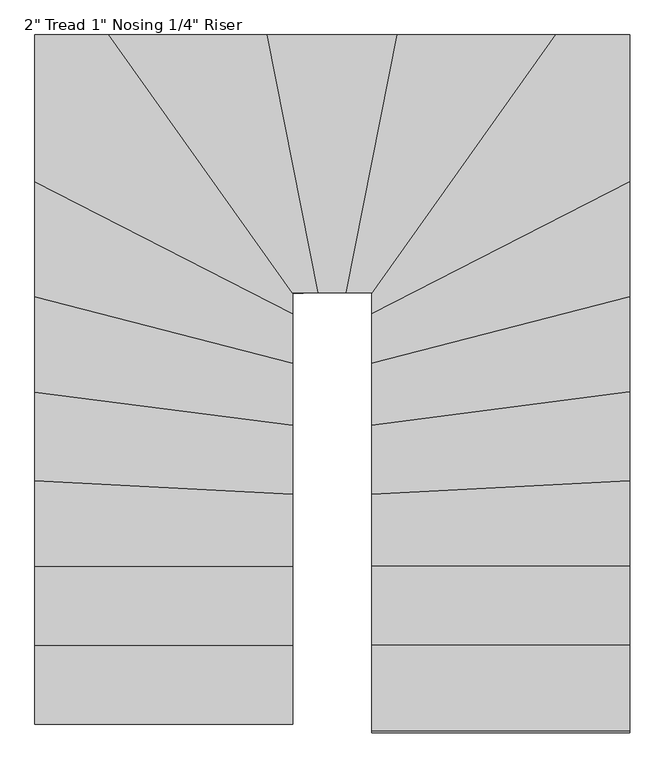
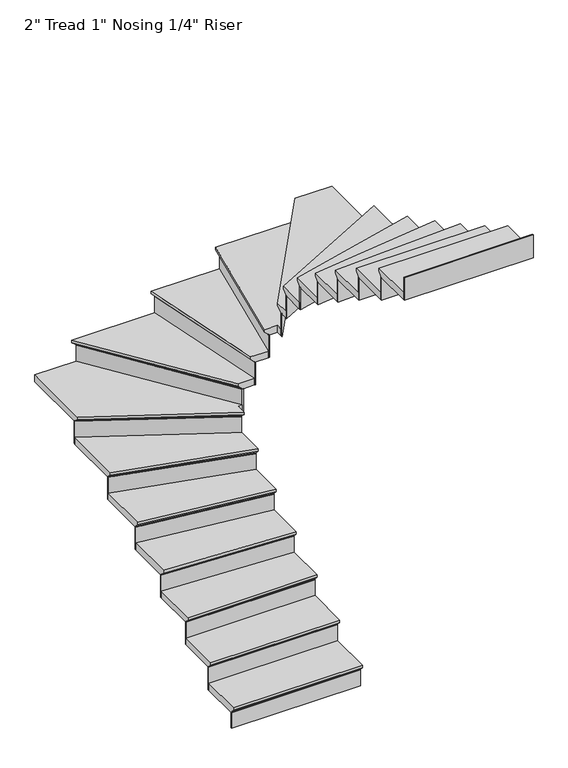
"""IFC4 building model written with IfcOpenShell, lengths in millimetres: stair flight geometry."""

from ifc_helpers import new_model, si_unit, origin, place, context, project, spatial, faceted_brep, source, transform, mapped, element, save


def stair_flight_f68c085a(model_context):
    return source(origin(), model_context, "Body", "Brep", [
        faceted_brep([(-12370.7568901, 792.321124, 150.2833333), (-12370.7568901, 792.321124, 169.3333333), (-13285.1568901, 792.321124, 169.3333333), (-13285.1568901, 792.321124, 150.2833333), (-12370.7568901, 817.721124, 124.8833333), (-13285.1568901, 817.721124, 124.8833333), (-12370.7568901, 1097.121124, 169.3333333), (-13285.1568901, 1097.121124, 169.3333333), (-13285.1568901, 817.721124, 118.5333333), (-13285.1568901, 1097.121124, 118.5333333), (-12370.7568901, 1097.121124, 118.5333333), (-12370.7568901, 817.721124, 118.5333333)], [[[0, 1, 2, 3]], [[4, 0, 3, 5]], [[2, 1, 6, 7]], [[8, 9, 10, 11]], [[2, 7, 9, 8, 5, 3]], [[8, 11, 4, 5]], [[6, 1, 0, 4, 11, 10]], [[7, 6, 10, 9]]]),
        faceted_brep([(-12370.7568901, 817.721124, 118.5333333), (-12370.7568901, 817.721124, 0.0), (-12370.7568901, 824.071124, 0.0), (-12370.7568901, 824.071124, 118.5333333), (-13285.1568901, 817.721124, 118.5333333), (-13285.1568901, 824.071124, 118.5333333), (-13285.1568901, 824.071124, 0.0), (-13285.1568901, 817.721124, 0.0)], [[[0, 1, 2, 3]], [[4, 5, 6, 7]], [[1, 0, 4, 7]], [[2, 1, 7, 6]], [[3, 2, 6, 5]], [[0, 3, 5, 4]]]),
        faceted_brep([(-12370.7568901, 1097.121124, 287.8666667), (-12370.7568901, 1097.121124, 118.5333333), (-12370.7568901, 1103.471124, 118.5333333), (-12370.7568901, 1103.471124, 287.8666667), (-13285.1568901, 1097.121124, 287.8666667), (-13285.1568901, 1103.471124, 287.8666667), (-13285.1568901, 1103.471124, 118.5333333), (-13285.1568901, 1097.121124, 118.5333333)], [[[0, 1, 2, 3]], [[4, 5, 6, 7]], [[1, 0, 4, 7]], [[2, 1, 7, 6]], [[3, 2, 6, 5]], [[0, 3, 5, 4]]]),
        faceted_brep([(-13285.1568901, 1071.721124, 338.6666667), (-12370.7568901, 1071.721124, 338.6666667), (-12370.7568901, 1376.521124, 338.6666667), (-13285.1568901, 1376.521124, 338.6666667), (-13285.1568901, 1097.121124, 287.8666667), (-13285.1568901, 1376.521124, 287.8666667), (-12370.7568901, 1376.521124, 287.8666667), (-12370.7568901, 1097.121124, 287.8666667), (-13285.1568901, 1097.121124, 294.2166667), (-13285.1568901, 1071.721124, 319.6166667), (-12370.7568901, 1097.121124, 294.2166667), (-12370.7568901, 1071.721124, 319.6166667)], [[[0, 1, 2, 3]], [[4, 5, 6, 7]], [[0, 3, 5, 4, 8, 9]], [[4, 7, 10, 8]], [[2, 1, 11, 10, 7, 6]], [[3, 2, 6, 5]], [[11, 1, 0, 9]], [[10, 11, 9, 8]]]),
        faceted_brep([(-12370.7568901, 1376.521124, 457.2), (-12370.7568901, 1376.521124, 287.8666667), (-12370.7568901, 1382.871124, 287.8666667), (-12370.7568901, 1382.871124, 457.2), (-13285.1568901, 1376.521124, 457.2), (-13285.1568901, 1382.871124, 457.2), (-13285.1568901, 1382.871124, 287.8666667), (-13285.1568901, 1376.521124, 287.8666667)], [[[0, 1, 2, 3]], [[4, 5, 6, 7]], [[1, 0, 4, 7]], [[2, 1, 7, 6]], [[3, 2, 6, 5]], [[0, 3, 5, 4]]]),
        faceted_brep([(-13285.1568901, 1351.121124, 508.0), (-12370.7568901, 1351.121124, 508.0), (-12370.7568901, 1632.1882855, 508.0), (-13285.1568901, 1679.7225559, 508.0), (-13285.1568901, 1376.521124, 457.2), (-13285.1568901, 1679.7225559, 457.2), (-12370.7568901, 1632.1882855, 457.2), (-12370.7568901, 1376.521124, 457.2), (-13285.1568901, 1376.521124, 463.55), (-13285.1568901, 1351.121124, 488.95), (-12370.7568901, 1376.521124, 463.55), (-12370.7568901, 1351.121124, 488.95)], [[[0, 1, 2, 3]], [[4, 5, 6, 7]], [[0, 3, 5, 4, 8, 9]], [[4, 7, 10, 8]], [[2, 1, 11, 10, 7, 6]], [[3, 2, 6, 5]], [[11, 1, 0, 9]], [[10, 11, 9, 8]]]),
        faceted_brep([(-12370.7568901, 1632.1882855, 626.5333333), (-12370.7568901, 1632.1882855, 457.2), (-12370.7568901, 1638.5468597, 457.2), (-12370.7568901, 1638.5468597, 626.5333333), (-13285.1568901, 1679.7225559, 626.5333333), (-13285.1568901, 1686.0811301, 626.5333333), (-13285.1568901, 1686.0811301, 457.2), (-13285.1568901, 1679.7225559, 457.2)], [[[0, 1, 2, 3]], [[4, 5, 6, 7]], [[1, 0, 4, 7]], [[2, 1, 7, 6]], [[3, 2, 6, 5]], [[0, 3, 5, 4]]]),
        faceted_brep([(-13285.1568901, 1654.2882592, 677.3333333), (-12370.7568901, 1606.7539888, 677.3333333), (-12370.7568901, 1876.3549853, 677.3333333), (-13285.1568901, 1994.711037, 677.3333333), (-13285.1568901, 1679.7225559, 626.5333333), (-13285.1568901, 1994.711037, 626.5333333), (-12370.7568901, 1876.3549853, 626.5333333), (-12370.7568901, 1632.1882855, 626.5333333), (-13285.1568901, 1679.7225559, 632.8833333), (-13285.1568901, 1654.2882592, 658.2833333), (-12370.7568901, 1632.1882855, 632.8833333), (-12370.7568901, 1606.7539888, 658.2833333)], [[[0, 1, 2, 3]], [[4, 5, 6, 7]], [[0, 3, 5, 4, 8, 9]], [[4, 7, 10, 8]], [[2, 1, 11, 10, 7, 6]], [[3, 2, 6, 5]], [[11, 1, 0, 9]], [[10, 11, 9, 8]]]),
        faceted_brep([(-12370.7568901, 1876.3549853, 795.8666667), (-12370.7568901, 1876.3549853, 626.5333333), (-12370.7568901, 1882.7579571, 626.5333333), (-12370.7568901, 1882.7579571, 795.8666667), (-13285.1568901, 1994.711037, 795.8666667), (-13285.1568901, 2001.1140088, 795.8666667), (-13285.1568901, 2001.1140088, 626.5333333), (-13285.1568901, 1994.711037, 626.5333333)], [[[0, 1, 2, 3]], [[4, 5, 6, 7]], [[1, 0, 4, 7]], [[2, 1, 7, 6]], [[3, 2, 6, 5]], [[0, 3, 5, 4]]]),
        faceted_brep([(-13285.1568901, 1969.0991499, 846.6666667), (-12370.7568901, 1850.7430982, 846.6666667), (-12370.7568901, 2097.9822078, 846.6666667), (-13285.1568901, 2333.1126552, 846.6666667), (-13285.1568901, 1994.711037, 795.8666667), (-13285.1568901, 2333.1126552, 795.8666667), (-12370.7568901, 2097.9822078, 795.8666667), (-12370.7568901, 1876.3549853, 795.8666667), (-13285.1568901, 1994.711037, 802.2166667), (-13285.1568901, 1969.0991499, 827.6166667), (-12370.7568901, 1876.3549853, 802.2166667), (-12370.7568901, 1850.7430982, 827.6166667)], [[[0, 1, 2, 3]], [[4, 5, 6, 7]], [[0, 3, 5, 4, 8, 9]], [[4, 7, 10, 8]], [[2, 1, 11, 10, 7, 6]], [[3, 2, 6, 5]], [[11, 1, 0, 9]], [[10, 11, 9, 8]]]),
        faceted_brep([(-12370.7568901, 2097.9822078, 965.2), (-12370.7568901, 2097.9822078, 795.8666667), (-12370.7568901, 2104.5387847, 795.8666667), (-12370.7568901, 2104.5387847, 965.2), (-13285.1568901, 2333.1126552, 965.2), (-13285.1568901, 2339.6692321, 965.2), (-13285.1568901, 2339.6692321, 795.8666667), (-13285.1568901, 2333.1126552, 795.8666667)], [[[0, 1, 2, 3]], [[4, 5, 6, 7]], [[1, 0, 4, 7]], [[2, 1, 7, 6]], [[3, 2, 6, 5]], [[0, 3, 5, 4]]]),
        faceted_brep([(-13285.1568901, 2306.8863477, 1016.0), (-12370.7568901, 2071.7559003, 1016.0), (-12370.7568901, 2274.3288439, 1016.0), (-13285.1568901, 2743.1534652, 1016.0), (-13285.1568901, 2333.1126552, 965.2), (-13285.1568901, 2743.1534652, 965.2), (-12370.7568901, 2274.3288439, 965.2), (-12370.7568901, 2097.9822078, 965.2), (-13285.1568901, 2333.1126552, 971.55), (-13285.1568901, 2306.8863477, 996.95), (-12370.7568901, 2097.9822078, 971.55), (-12370.7568901, 2071.7559003, 996.95)], [[[0, 1, 2, 3]], [[4, 5, 6, 7]], [[0, 3, 5, 4, 8, 9]], [[4, 7, 10, 8]], [[2, 1, 11, 10, 7, 6]], [[3, 2, 6, 5]], [[11, 1, 0, 9]], [[10, 11, 9, 8]]]),
        faceted_brep([(-12370.7568901, 2274.3288439, 1134.5333333), (-12370.7568901, 2274.3288439, 965.2), (-12370.7568901, 2281.464827, 965.2), (-12370.7568901, 2281.464827, 1134.5333333), (-13285.1568901, 2743.1534652, 1134.5333333), (-13285.1568901, 2750.2894483, 1134.5333333), (-13285.1568901, 2750.2894483, 965.2), (-13285.1568901, 2743.1534652, 965.2)], [[[0, 1, 2, 3]], [[4, 5, 6, 7]], [[1, 0, 4, 7]], [[2, 1, 7, 6]], [[3, 2, 6, 5]], [[0, 3, 5, 4]]]),
        faceted_brep([(-12991.4757564, 3234.4528159, 1185.3333333), (-13285.1568901, 3234.4528159, 1185.3333333), (-13285.1568901, 2714.6095327, 1185.3333333), (-12370.7568901, 2245.7849113, 1185.3333333), (-12370.7568901, 2320.0528159, 1185.3333333), (-12341.2018072, 2320.0528159, 1185.3333333), (-13285.1568901, 3234.4528159, 1134.5333333), (-12991.4757564, 3234.4528159, 1134.5333333), (-12341.2018072, 2320.0528159, 1134.5333333), (-12370.7568901, 2320.0528159, 1134.5333333), (-12370.7568901, 2274.3288439, 1134.5333333), (-13285.1568901, 2743.1534652, 1134.5333333), (-13285.1568901, 2743.1534652, 1140.8833333), (-13285.1568901, 2714.6095327, 1166.2833333), (-12370.7568901, 2274.3288439, 1140.8833333), (-12370.7568901, 2245.7849113, 1166.2833333)], [[[0, 1, 2, 3, 4, 5]], [[6, 7, 8, 9, 10, 11]], [[1, 0, 7, 6]], [[2, 1, 6, 11, 12, 13]], [[11, 10, 14, 12]], [[4, 3, 15, 14, 10, 9]], [[5, 4, 9, 8]], [[0, 5, 8, 7]], [[15, 3, 2, 13]], [[14, 15, 13, 12]]]),
        faceted_brep([(-12341.2018072, 2320.0528159, 1303.8666667), (-12341.2018072, 2320.0528159, 1134.5333333), (-12333.4098325, 2320.0528159, 1134.5333333), (-12333.4098325, 2320.0528159, 1303.8666667), (-12991.4757564, 3234.4528159, 1303.8666667), (-12983.6837816, 3234.4528159, 1303.8666667), (-12983.6837816, 3234.4528159, 1134.5333333), (-12991.4757564, 3234.4528159, 1134.5333333)], [[[0, 1, 2, 3]], [[4, 5, 6, 7]], [[1, 0, 4, 7]], [[2, 1, 7, 6]], [[3, 2, 6, 5]], [[0, 3, 5, 4]]]),
        faceted_brep([(-13022.6436556, 3234.4528159, 1354.6666667), (-12372.3697064, 2320.0528159, 1354.6666667), (-12254.7477202, 2320.0528159, 1354.6666667), (-12434.9885765, 3234.4528159, 1354.6666667), (-12991.4757564, 3234.4528159, 1303.8666667), (-12434.9885765, 3234.4528159, 1303.8666667), (-12254.7477202, 2320.0528159, 1303.8666667), (-12341.2018072, 2320.0528159, 1303.8666667), (-12991.4757564, 3234.4528159, 1310.2166667), (-13022.6436556, 3234.4528159, 1335.6166667), (-12341.2018072, 2320.0528159, 1310.2166667), (-12372.3697064, 2320.0528159, 1335.6166667)], [[[0, 1, 2, 3]], [[4, 5, 6, 7]], [[0, 3, 5, 4, 8, 9]], [[4, 7, 10, 8]], [[2, 1, 11, 10, 7, 6]], [[3, 2, 6, 5]], [[11, 1, 0, 9]], [[10, 11, 9, 8]]]),
        faceted_brep([(-12254.7477202, 2320.0528159, 1473.2), (-12254.7477202, 2320.0528159, 1303.8666667), (-12248.2755347, 2320.0528159, 1303.8666667), (-12248.2755347, 2320.0528159, 1473.2), (-12434.9885765, 3234.4528159, 1473.2), (-12428.5163911, 3234.4528159, 1473.2), (-12428.5163911, 3234.4528159, 1303.8666667), (-12434.9885765, 3234.4528159, 1303.8666667)], [[[0, 1, 2, 3]], [[4, 5, 6, 7]], [[1, 0, 4, 7]], [[2, 1, 7, 6]], [[3, 2, 6, 5]], [[0, 3, 5, 4]]]),
        faceted_brep([(-12460.8773183, 3234.4528159, 1524.0), (-12280.6364619, 2320.0528159, 1524.0), (-12155.5885765, 2320.0528159, 1524.0), (-11975.3477202, 3234.4528159, 1524.0), (-12434.9885765, 3234.4528159, 1473.2), (-11975.3477202, 3234.4528159, 1473.2), (-12155.5885765, 2320.0528159, 1473.2), (-12254.7477202, 2320.0528159, 1473.2), (-12434.9885765, 3234.4528159, 1479.55), (-12460.8773183, 3234.4528159, 1504.95), (-12254.7477202, 2320.0528159, 1479.55), (-12280.6364619, 2320.0528159, 1504.95)], [[[0, 1, 2, 3]], [[4, 5, 6, 7]], [[0, 3, 5, 4, 8, 9]], [[4, 7, 10, 8]], [[2, 1, 11, 10, 7, 6]], [[3, 2, 6, 5]], [[11, 1, 0, 9]], [[10, 11, 9, 8]]]),
        faceted_brep([(-12155.5885765, 2320.0528159, 1642.5333333), (-12155.5885765, 2320.0528159, 1473.2), (-12149.1163911, 2320.0528159, 1473.2), (-12149.1163911, 2320.0528159, 1642.5333333), (-11975.3477202, 3234.4528159, 1642.5333333), (-11968.8755347, 3234.4528159, 1642.5333333), (-11968.8755347, 3234.4528159, 1473.2), (-11975.3477202, 3234.4528159, 1473.2)], [[[0, 1, 2, 3]], [[4, 5, 6, 7]], [[1, 0, 4, 7]], [[2, 1, 7, 6]], [[3, 2, 6, 5]], [[0, 3, 5, 4]]]),
        faceted_brep([(-12001.2364619, 3234.4528159, 1693.3333333), (-12181.4773183, 2320.0528159, 1693.3333333), (-12091.3568901, 2320.0528159, 1693.3333333), (-12091.3568901, 2273.9573414, 1693.3333333), (-11408.3022254, 3234.4528159, 1693.3333333), (-11975.3477202, 3234.4528159, 1642.5333333), (-11408.3022254, 3234.4528159, 1642.5333333), (-12091.3568901, 2273.9573414, 1642.5333333), (-12091.3568901, 2320.0528159, 1642.5333333), (-12155.5885765, 2320.0528159, 1642.5333333), (-11975.3477202, 3234.4528159, 1648.8833333), (-12001.2364619, 3234.4528159, 1674.2833333), (-12155.5885765, 2320.0528159, 1648.8833333), (-12181.4773183, 2320.0528159, 1674.2833333)], [[[0, 1, 2, 3, 4]], [[5, 6, 7, 8, 9]], [[0, 4, 6, 5, 10, 11]], [[5, 9, 12, 10]], [[2, 1, 13, 12, 9, 8]], [[3, 2, 8, 7]], [[4, 3, 7, 6]], [[13, 1, 0, 11]], [[12, 13, 11, 10]]]),
        faceted_brep([(-12091.3568901, 2273.9573414, 1811.8666667), (-12091.3568901, 2273.9573414, 1642.5333333), (-12091.3568901, 2263.0004489, 1642.5333333), (-12091.3568901, 2263.0004489, 1811.8666667), (-11408.3022254, 3234.4528159, 1811.8666667), (-11400.5102506, 3234.4528159, 1811.8666667), (-11400.5102506, 3234.4528159, 1642.5333333), (-11408.3022254, 3234.4528159, 1642.5333333)], [[[0, 1, 2, 3]], [[4, 5, 6, 7]], [[1, 0, 4, 7]], [[2, 1, 7, 6]], [[3, 2, 6, 5]], [[0, 3, 5, 4]]]),
        faceted_brep([(-11176.9568901, 2686.0656001, 1862.6666667), (-11176.9568901, 3234.4528159, 1862.6666667), (-11439.4701246, 3234.4528159, 1862.6666667), (-12091.3568901, 2317.7849113, 1862.6666667), (-12091.3568901, 2217.2409788, 1862.6666667), (-11176.9568901, 3234.4528159, 1811.8666667), (-11176.9568901, 2686.0656001, 1811.8666667), (-12091.3568901, 2217.2409788, 1811.8666667), (-12091.3568901, 2273.9573414, 1811.8666667), (-11408.3022254, 3234.4528159, 1811.8666667), (-11408.3022254, 3234.4528159, 1818.2166667), (-11439.4701246, 3234.4528159, 1843.6166667), (-12091.3568901, 2273.9573414, 1818.2166667), (-12091.3568901, 2317.7849113, 1843.6166667)], [[[0, 1, 2, 3, 4]], [[5, 6, 7, 8, 9]], [[1, 0, 6, 5]], [[2, 1, 5, 9, 10, 11]], [[9, 8, 12, 10]], [[4, 3, 13, 12, 8, 7]], [[0, 4, 7, 6]], [[13, 3, 2, 11]], [[12, 13, 11, 10]]]),
        faceted_brep([(-12091.3568901, 2217.2409788, 1981.2), (-12091.3568901, 2217.2409788, 1811.8666667), (-12091.3568901, 2210.1049957, 1811.8666667), (-12091.3568901, 2210.1049957, 1981.2), (-11176.9568901, 2686.0656001, 1981.2), (-11176.9568901, 2678.929617, 1981.2), (-11176.9568901, 2678.929617, 1811.8666667), (-11176.9568901, 2686.0656001, 1811.8666667)], [[[0, 1, 2, 3]], [[4, 5, 6, 7]], [[1, 0, 4, 7]], [[2, 1, 7, 6]], [[3, 2, 6, 5]], [[0, 3, 5, 4]]]),
        faceted_brep([(-11176.9568901, 2714.6095327, 2032.0), (-12091.3568901, 2245.7849113, 2032.0), (-12091.3568901, 2045.5295929, 2032.0), (-11176.9568901, 2280.6600403, 2032.0), (-11176.9568901, 2686.0656001, 1981.2), (-11176.9568901, 2280.6600403, 1981.2), (-12091.3568901, 2045.5295929, 1981.2), (-12091.3568901, 2217.2409788, 1981.2), (-11176.9568901, 2686.0656001, 1987.55), (-11176.9568901, 2714.6095327, 2012.95), (-12091.3568901, 2217.2409788, 1987.55), (-12091.3568901, 2245.7849113, 2012.95)], [[[0, 1, 2, 3]], [[4, 5, 6, 7]], [[0, 3, 5, 4, 8, 9]], [[4, 7, 10, 8]], [[2, 1, 11, 10, 7, 6]], [[3, 2, 6, 5]], [[11, 1, 0, 9]], [[10, 11, 9, 8]]]),
        faceted_brep([(-12091.3568901, 2045.5295929, 2150.5333333), (-12091.3568901, 2045.5295929, 1981.2), (-12091.3568901, 2038.973016, 1981.2), (-12091.3568901, 2038.973016, 2150.5333333), (-11176.9568901, 2280.6600403, 2150.5333333), (-11176.9568901, 2274.1034634, 2150.5333333), (-11176.9568901, 2274.1034634, 1981.2), (-11176.9568901, 2280.6600403, 1981.2)], [[[0, 1, 2, 3]], [[4, 5, 6, 7]], [[1, 0, 4, 7]], [[2, 1, 7, 6]], [[3, 2, 6, 5]], [[0, 3, 5, 4]]]),
        faceted_brep([(-11176.9568901, 2306.8863477, 2201.3333333), (-12091.3568901, 2071.7559003, 2201.3333333), (-12091.3568901, 1825.1312111, 2201.3333333), (-11176.9568901, 1943.4872628, 2201.3333333), (-11176.9568901, 2280.6600403, 2150.5333333), (-11176.9568901, 1943.4872628, 2150.5333333), (-12091.3568901, 1825.1312111, 2150.5333333), (-12091.3568901, 2045.5295929, 2150.5333333), (-11176.9568901, 2280.6600403, 2156.8833333), (-11176.9568901, 2306.8863477, 2182.2833333), (-12091.3568901, 2045.5295929, 2156.8833333), (-12091.3568901, 2071.7559003, 2182.2833333)], [[[0, 1, 2, 3]], [[4, 5, 6, 7]], [[0, 3, 5, 4, 8, 9]], [[4, 7, 10, 8]], [[2, 1, 11, 10, 7, 6]], [[3, 2, 6, 5]], [[11, 1, 0, 9]], [[10, 11, 9, 8]]]),
        faceted_brep([(-12091.3568901, 1825.1312111, 2319.8666667), (-12091.3568901, 1825.1312111, 2150.5333333), (-12091.3568901, 1818.7282393, 2150.5333333), (-12091.3568901, 1818.7282393, 2319.8666667), (-11176.9568901, 1943.4872628, 2319.8666667), (-11176.9568901, 1937.084291, 2319.8666667), (-11176.9568901, 1937.084291, 2150.5333333), (-11176.9568901, 1943.4872628, 2150.5333333)], [[[0, 1, 2, 3]], [[4, 5, 6, 7]], [[1, 0, 4, 7]], [[2, 1, 7, 6]], [[3, 2, 6, 5]], [[0, 3, 5, 4]]]),
        faceted_brep([(-11176.9568901, 1969.0991499, 2370.6666667), (-12091.3568901, 1850.7430982, 2370.6666667), (-12091.3568901, 1581.3196922, 2370.6666667), (-11176.9568901, 1628.8539626, 2370.6666667), (-11176.9568901, 1943.4872628, 2319.8666667), (-11176.9568901, 1628.8539626, 2319.8666667), (-12091.3568901, 1581.3196922, 2319.8666667), (-12091.3568901, 1825.1312111, 2319.8666667), (-11176.9568901, 1943.4872628, 2326.2166667), (-11176.9568901, 1969.0991499, 2351.6166667), (-12091.3568901, 1825.1312111, 2326.2166667), (-12091.3568901, 1850.7430982, 2351.6166667)], [[[0, 1, 2, 3]], [[4, 5, 6, 7]], [[0, 3, 5, 4, 8, 9]], [[4, 7, 10, 8]], [[2, 1, 11, 10, 7, 6]], [[3, 2, 6, 5]], [[11, 1, 0, 9]], [[10, 11, 9, 8]]]),
        faceted_brep([(-12091.3568901, 1581.3196922, 2489.2), (-12091.3568901, 1581.3196922, 2319.8666667), (-12091.3568901, 1574.961118, 2319.8666667), (-12091.3568901, 1574.961118, 2489.2), (-11176.9568901, 1628.8539626, 2489.2), (-11176.9568901, 1622.4953884, 2489.2), (-11176.9568901, 1622.4953884, 2319.8666667), (-11176.9568901, 1628.8539626, 2319.8666667)], [[[0, 1, 2, 3]], [[4, 5, 6, 7]], [[1, 0, 4, 7]], [[2, 1, 7, 6]], [[3, 2, 6, 5]], [[0, 3, 5, 4]]]),
        faceted_brep([(-11176.9568901, 1654.2882592, 2540.0), (-12091.3568901, 1606.7539888, 2540.0), (-12091.3568901, 1325.721124, 2540.0), (-11176.9568901, 1325.721124, 2540.0), (-11176.9568901, 1628.8539626, 2489.2), (-11176.9568901, 1325.721124, 2489.2), (-12091.3568901, 1325.721124, 2489.2), (-12091.3568901, 1581.3196922, 2489.2), (-11176.9568901, 1628.8539626, 2495.55), (-11176.9568901, 1654.2882592, 2520.95), (-12091.3568901, 1581.3196922, 2495.55), (-12091.3568901, 1606.7539888, 2520.95)], [[[0, 1, 2, 3]], [[4, 5, 6, 7]], [[0, 3, 5, 4, 8, 9]], [[4, 7, 10, 8]], [[2, 1, 11, 10, 7, 6]], [[3, 2, 6, 5]], [[11, 1, 0, 9]], [[10, 11, 9, 8]]]),
        faceted_brep([(-12091.3568901, 1325.721124, 2658.5333333), (-12091.3568901, 1325.721124, 2489.2), (-12091.3568901, 1319.371124, 2489.2), (-12091.3568901, 1319.371124, 2658.5333333), (-11176.9568901, 1325.721124, 2658.5333333), (-11176.9568901, 1319.371124, 2658.5333333), (-11176.9568901, 1319.371124, 2489.2), (-11176.9568901, 1325.721124, 2489.2)], [[[0, 1, 2, 3]], [[4, 5, 6, 7]], [[1, 0, 4, 7]], [[2, 1, 7, 6]], [[3, 2, 6, 5]], [[0, 3, 5, 4]]]),
        faceted_brep([(-11176.9568901, 1351.121124, 2709.3333333), (-12091.3568901, 1351.121124, 2709.3333333), (-12091.3568901, 1046.321124, 2709.3333333), (-11176.9568901, 1046.321124, 2709.3333333), (-11176.9568901, 1325.721124, 2658.5333333), (-11176.9568901, 1046.321124, 2658.5333333), (-12091.3568901, 1046.321124, 2658.5333333), (-12091.3568901, 1325.721124, 2658.5333333), (-11176.9568901, 1325.721124, 2664.8833333), (-11176.9568901, 1351.121124, 2690.2833333), (-12091.3568901, 1325.721124, 2664.8833333), (-12091.3568901, 1351.121124, 2690.2833333)], [[[0, 1, 2, 3]], [[4, 5, 6, 7]], [[0, 3, 5, 4, 8, 9]], [[4, 7, 10, 8]], [[2, 1, 11, 10, 7, 6]], [[3, 2, 6, 5]], [[11, 1, 0, 9]], [[10, 11, 9, 8]]]),
        faceted_brep([(-12091.3568901, 1046.321124, 2827.8666667), (-12091.3568901, 1046.321124, 2658.5333333), (-12091.3568901, 1039.971124, 2658.5333333), (-12091.3568901, 1039.971124, 2827.8666667), (-11176.9568901, 1046.321124, 2827.8666667), (-11176.9568901, 1039.971124, 2827.8666667), (-11176.9568901, 1039.971124, 2658.5333333), (-11176.9568901, 1046.321124, 2658.5333333)], [[[0, 1, 2, 3]], [[4, 5, 6, 7]], [[1, 0, 4, 7]], [[2, 1, 7, 6]], [[3, 2, 6, 5]], [[0, 3, 5, 4]]]),
        faceted_brep([(-12091.3568901, 766.921124, 2997.2), (-12091.3568901, 766.921124, 2827.8666667), (-12091.3568901, 760.571124, 2827.8666667), (-12091.3568901, 760.571124, 2997.2), (-11176.9568901, 766.921124, 2997.2), (-11176.9568901, 760.571124, 2997.2), (-11176.9568901, 760.571124, 2827.8666667), (-11176.9568901, 766.921124, 2827.8666667)], [[[0, 1, 2, 3]], [[4, 5, 6, 7]], [[1, 0, 4, 7]], [[2, 1, 7, 6]], [[3, 2, 6, 5]], [[0, 3, 5, 4]]]),
        faceted_brep([(-11176.9568901, 1071.721124, 2878.6666667), (-12091.3568901, 1071.721124, 2878.6666667), (-12091.3568901, 766.921124, 2878.6666667), (-11176.9568901, 766.921124, 2878.6666667), (-11176.9568901, 1046.321124, 2827.8666667), (-11176.9568901, 766.921124, 2827.8666667), (-12091.3568901, 766.921124, 2827.8666667), (-12091.3568901, 1046.321124, 2827.8666667), (-11176.9568901, 1046.321124, 2834.2166667), (-11176.9568901, 1071.721124, 2859.6166667), (-12091.3568901, 1046.321124, 2834.2166667), (-12091.3568901, 1071.721124, 2859.6166667)], [[[0, 1, 2, 3]], [[4, 5, 6, 7]], [[0, 3, 5, 4, 8, 9]], [[4, 7, 10, 8]], [[2, 1, 11, 10, 7, 6]], [[3, 2, 6, 5]], [[11, 1, 0, 9]], [[10, 11, 9, 8]]]),
    ])


if __name__ == "__main__":
    model = new_model("IFC4")
    model_context = context("Model", 3, world=origin())
    ifc_project = project(units=[si_unit("LENGTHUNIT", "METRE", prefix="MILLI")], contexts=[model_context])
    site = spatial("IfcSite", under=ifc_project)
    building = spatial("IfcBuilding", under=site)
    placement = place(None, origin())
    stair_flight_shape = stair_flight_f68c085a(model_context)
    element("IfcStairFlight", 1, ObjectType="2\" Tread 1\" Nosing 1/4\" Riser", at=placement, inside=building, context=model_context, shape_type="MappedRepresentation", body=[
        mapped(stair_flight_shape, transform((0.0, 0.0, 0.0), x_axis=(1.0, 0.0, 0.0), y_axis=(0.0, 1.0, 0.0), z_axis=(0.0, 0.0, 1.0))),
    ])
    save(model, "model.ifc")
